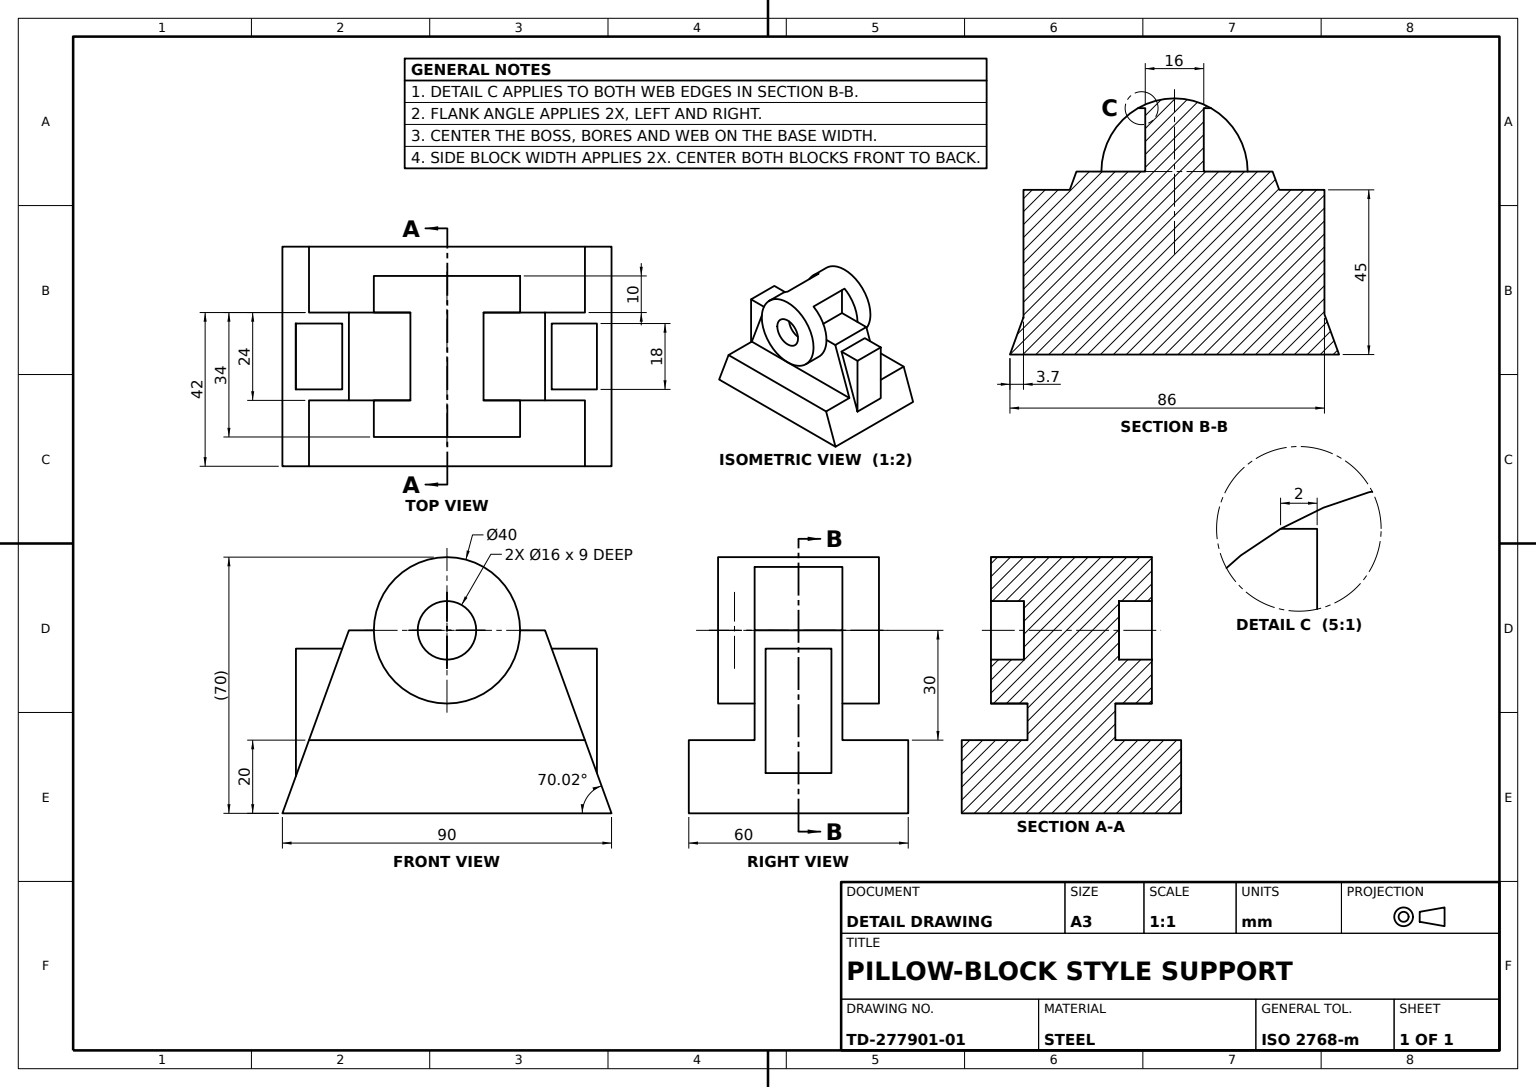
from build123d import *

# Parameters (mm, degrees)
BASE_TRAPEZOID_SKETCH_W     = 90
BASE_TRAPEZOID_SKETCH_H     = 20
TRAPEZOID_BASE_DEPTH        = 60
CYLINDER_SUPPORT_DEPTH      = 42
SUPPORT_NOTCH_CUT_DEPTH     = 18
SUPPORT_RELIEF_CUT_DEPTH    = 24
THROUGH_PROFILE_CUT_DEPTH   = 60
CYLINDER_SKETCH_40_R        = 20
CYLINDER_40_DEPTH           = 34
CYLINDER_START              = 10
CYLINDER_EXTENSION_SKETCH_R = 20
CYLINDER_EXTENSION_40_DEPTH = 10
FRONT_BORE_SKETCH_16_R      = 8
FRONT_BORE_16_DEPTH         = 10
REAR_START                  = -10
REAR_BORE_SKETCH_R          = 8
REAR_BORE_DEPTH             = 10
SIDE_BLOCKS_DEPTH           = 86
BLOCK_TRIM_SKETCH_W         = 18
BLOCK_TRIM_SKETCH_H         = 35
BLOCK_TRIM_CUT_DEPTH        = 3.7
SLOT_A_SKETCH_W             = 24
SLOT_A_SKETCH_H             = 20
SLOT_A_CUT_DEPTH            = 10
SLOT_B_SKETCH_W             = 24
SLOT_B_SKETCH_H             = 20
SLOT_B_CUT_DEPTH            = 10
FRONT_START                 = 10
FRONT_BORE_FILL_SKETCH_R    = 8
FRONT_BORE_FILL_DEPTH       = 10
REAR_BORE_FILL_SKETCH_R     = 8
REAR_BORE_FILL_DEPTH        = 10
SLOT_B_FLOOR_SKETCH_W       = 24
SLOT_B_FLOOR_SKETCH_H       = 17.320508076
SLOT_B_FLOOR_CUT_DEPTH      = 2
SLOT_A_FLOOR_SKETCH_W       = 24
SLOT_A_FLOOR_SKETCH_H       = 17.320508076
SLOT_A_FLOOR_CUT_DEPTH      = 2
FRONT_BORE_RECUT_SKETCH_R   = 8
FRONT_BORE_RECUT_DEPTH      = 9
REAR_START_2                = -9
REAR_BORE_RECUT_SKETCH_R    = 8
REAR_BORE_RECUT_DEPTH       = 9


with BuildPart() as part:
    # Base Trapezoid Sketch → Trapezoid Base (new body)
    with BuildSketch(Plane.XY):
        with Locations((45, 10)):
            Rectangle(BASE_TRAPEZOID_SKETCH_W, BASE_TRAPEZOID_SKETCH_H)
    extrude(amount=TRAPEZOID_BASE_DEPTH)

    # Support Profile Sketch → Cylinder Support (add)
    with BuildSketch(Plane.XY.offset(60)):
        Polygon((45, 20), (7.272727273, 20), (20, 55), (45, 55), (70, 55), (82.727272727, 20), align=None)
    extrude(amount=-CYLINDER_SUPPORT_DEPTH)

    # Support Notch Sketch → Support Notch Cut (cut)
    with BuildSketch(Plane.XY.offset(60)):
        Polygon((7.272727273, 20), (20, 55), (70, 55), (82.727272727, 20), align=None)
    extrude(amount=-SUPPORT_NOTCH_CUT_DEPTH, mode=Mode.SUBTRACT)

    # Support Relief Sketch → Support Relief Cut (cut)
    with BuildSketch(Plane.XY.offset(42)):
        Polygon((45, 50), (71.818181818, 50), (70, 55), (20, 55), (18.181818182, 50), align=None)
    extrude(amount=-SUPPORT_RELIEF_CUT_DEPTH, mode=Mode.SUBTRACT)

    # Through Profile Sketch → Through Profile Cut (cut)
    with BuildSketch(Plane.XY.offset(60)):
        Polygon((7.272727273, 20), (0, 20), (0, 0), align=None)
        Polygon((90, 20), (82.727272727, 20), (90, 0), align=None)
    extrude(amount=-THROUGH_PROFILE_CUT_DEPTH, mode=Mode.SUBTRACT)

    # Cylinder Sketch Ø40 → Cylinder Ø40 (add)
    with BuildSketch(Plane.XY.offset(42)):
        with Locations((45, 50)):
            Circle(CYLINDER_SKETCH_40_R)
    extrude(amount=-CYLINDER_40_DEPTH)

    # Cylinder Extension Sketch → Cylinder Extension Ø40 (add)
    with BuildSketch(Plane.XY.offset(42).offset(CYLINDER_START)):
        with Locations((45, 50)):
            Circle(CYLINDER_EXTENSION_SKETCH_R)
    extrude(amount=-CYLINDER_EXTENSION_40_DEPTH)

    # Front Bore Sketch Ø16 → Front Bore Ø16 (cut)
    with BuildSketch(Plane.XY.offset(52)):
        with Locations((45, 50)):
            Circle(FRONT_BORE_SKETCH_16_R)
    extrude(amount=-FRONT_BORE_16_DEPTH, mode=Mode.SUBTRACT)

    # Rear Bore Sketch → Rear Bore (cut)
    with BuildSketch(Plane(origin=(0, 0, 8), x_dir=(-1, 0, 0), z_dir=(0, 0, -1)).offset(REAR_START)):
        with Locations(Location((-45, 50, 0), (0, 0, 180))):
            Circle(REAR_BORE_SKETCH_R)
    extrude(amount=REAR_BORE_DEPTH, mode=Mode.SUBTRACT)

    # Side Block Sketch → Side Blocks (add)
    with BuildSketch(Plane(origin=(0, 0, 0), x_dir=(0, 0, -1), z_dir=(1, 0, 0))):
        Polygon((-30, 45), (-39, 45), (-39, 10), (-21, 10), (-21, 45), align=None)
    extrude(amount=SIDE_BLOCKS_DEPTH)

    # Block Trim Sketch → Block Trim Cut (cut)
    with BuildSketch(Plane.ZY):
        with Locations((30, 27.5)):
            Rectangle(BLOCK_TRIM_SKETCH_W, BLOCK_TRIM_SKETCH_H)
    extrude(amount=-BLOCK_TRIM_CUT_DEPTH, mode=Mode.SUBTRACT)

    # Slot A Sketch → Slot A Cut (cut)
    with BuildSketch(Plane(origin=(65, 0, 0), x_dir=(0, 0, -1), z_dir=(1, 0, 0))):
        with Locations((-30, 60)):
            Rectangle(SLOT_A_SKETCH_W, SLOT_A_SKETCH_H)
    extrude(amount=-SLOT_A_CUT_DEPTH, mode=Mode.SUBTRACT)

    # Slot B Sketch → Slot B Cut (cut)
    with BuildSketch(Plane(origin=(25, 0, 0), x_dir=(0, 0, -1), z_dir=(1, 0, 0))):
        with Locations((-30, 60)):
            Rectangle(SLOT_B_SKETCH_W, SLOT_B_SKETCH_H)
    extrude(amount=SLOT_B_CUT_DEPTH, mode=Mode.SUBTRACT)

    # Front Bore Fill Sketch → Front Bore Fill (add)
    with BuildSketch(Plane.XY.offset(42).offset(FRONT_START)):
        with Locations(Location((45, 50, 0), (0, 0, 180))):
            Circle(FRONT_BORE_FILL_SKETCH_R)
    extrude(amount=-FRONT_BORE_FILL_DEPTH)

    # Rear Bore Fill Sketch → Rear Bore Fill (add)
    with BuildSketch(Plane(origin=(0, 0, 18), x_dir=(-1, 0, 0), z_dir=(0, 0, -1))):
        with Locations((-45, 50)):
            Circle(REAR_BORE_FILL_SKETCH_R)
    extrude(amount=REAR_BORE_FILL_DEPTH)

    # Slot B Floor Sketch → Slot B Floor Cut (cut)
    with BuildSketch(Plane.ZY.offset(-35)):
        with Locations((30, 58.660254038)):
            Rectangle(SLOT_B_FLOOR_SKETCH_W, SLOT_B_FLOOR_SKETCH_H)
    extrude(amount=-SLOT_B_FLOOR_CUT_DEPTH, mode=Mode.SUBTRACT)

    # Slot A Floor Sketch → Slot A Floor Cut (cut)
    with BuildSketch(Plane(origin=(55, 0, 0), x_dir=(0, 0, -1), z_dir=(1, 0, 0))):
        with Locations((-30, 58.660254038)):
            Rectangle(SLOT_A_FLOOR_SKETCH_W, SLOT_A_FLOOR_SKETCH_H)
    extrude(amount=-SLOT_A_FLOOR_CUT_DEPTH, mode=Mode.SUBTRACT)

    # Front Bore Recut Sketch → Front Bore Recut (cut)
    with BuildSketch(Plane.XY.offset(52)):
        with Locations((45, 50)):
            Circle(FRONT_BORE_RECUT_SKETCH_R)
    extrude(amount=-FRONT_BORE_RECUT_DEPTH, mode=Mode.SUBTRACT)

    # Rear Bore Recut Sketch → Rear Bore Recut (cut)
    with BuildSketch(Plane(origin=(0, 0, 8), x_dir=(-1, 0, 0), z_dir=(0, 0, -1)).offset(REAR_START_2)):
        with Locations(Location((-45, 50, 0), (0, 0, 180))):
            Circle(REAR_BORE_RECUT_SKETCH_R)
    extrude(amount=REAR_BORE_RECUT_DEPTH, mode=Mode.SUBTRACT)


solid = part.part
